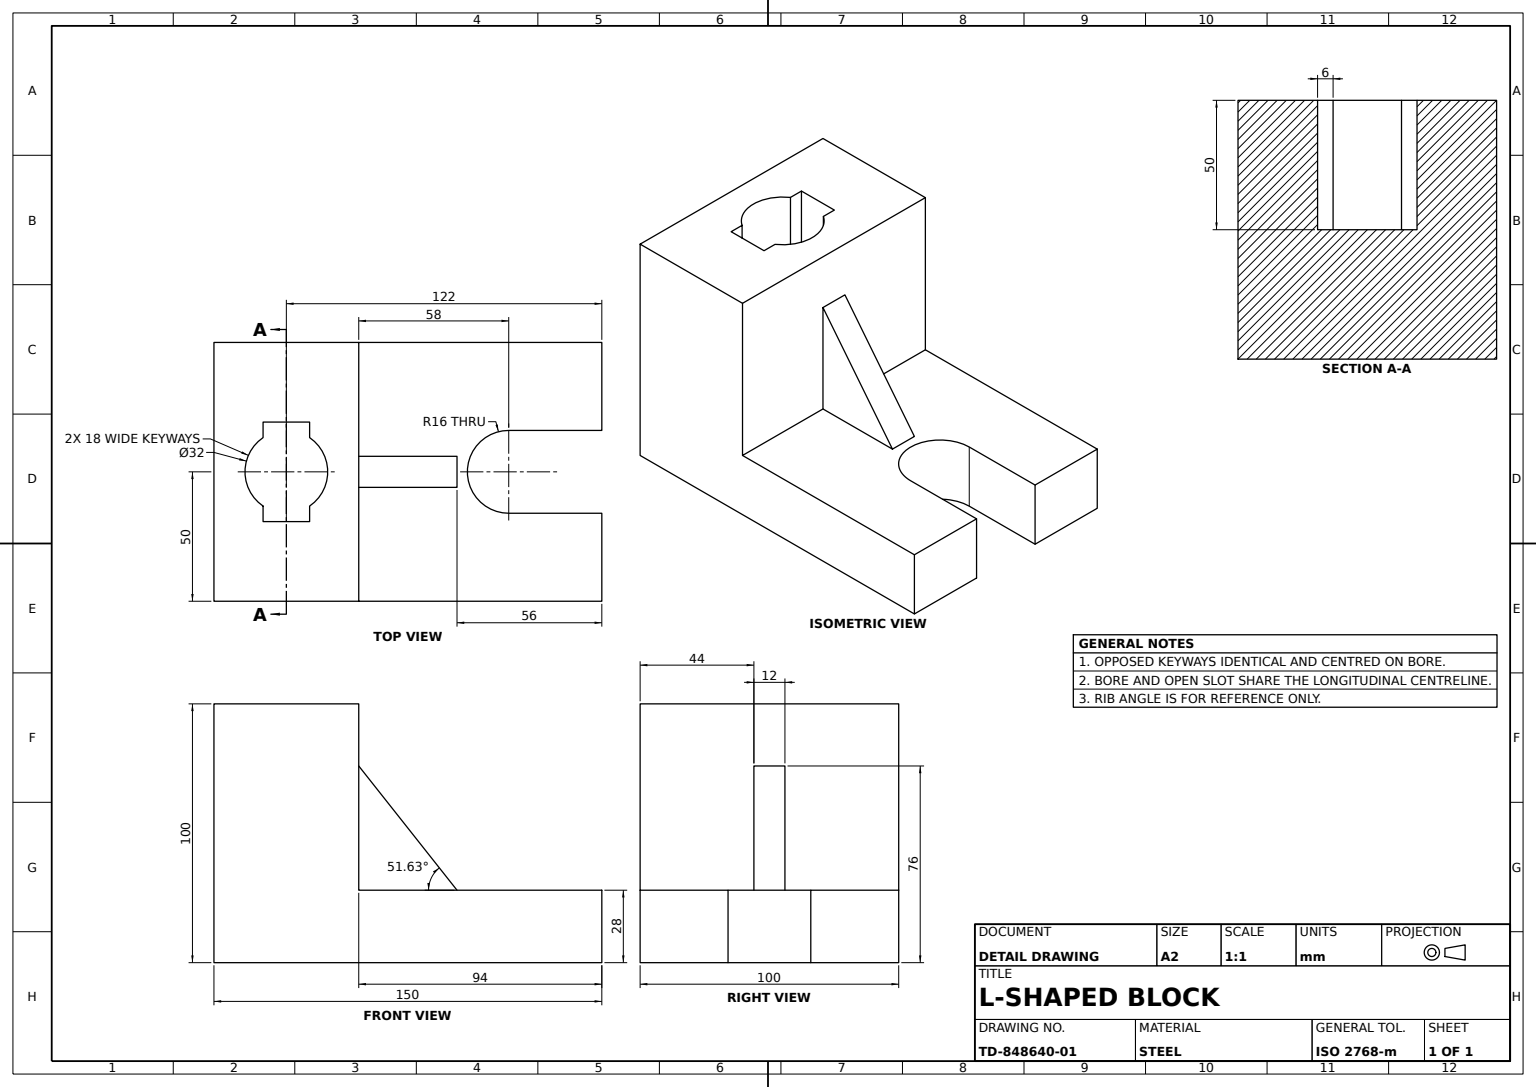
SolidWorks part; units mm, degrees
material "Plain Carbon Steel"
ref_plane "Front Plane" through (0, 0, 0) normal (0, 0, 1) x (1, 0, 0)
ref_plane "Top Plane" through (0, 0, 0) normal (0, 1, 0) x (1, 0, 0)
ref_plane "Right Plane" through (0, 0, 0) normal (1, 0, 0) x (0, 0, -1)
sketch "L-Block Profile Sketch" plane through (0, 0, 0) normal (0, 0, 1) x (1, 0, 0)
  line L0 (0, 0) -> (150, 0)
  line L1 (150, 0) -> (150, 100)
  line L2 (150, 100) -> (94, 100)
  line L3 (0, 0) -> (0, 28)
  line L4 (0, 28) -> (94, 28)
  line L5 (94, 28) -> (94, 100)
  dimension "D1" = 94
  dimension "D2" = 150
  dimension "D3" = 28
  dimension "D4" = 100
extrude "L-Block Base" add sketch "L-Block Profile Sketch" along normal blind 100
sketch "Keyed Bore Sketch" plane through (0, 100, 0) normal (0, 1, 0) x (1, 0, 0)
  line L0 (113, -69.2288) -> (131, -69.2288)
  line L5 (113, -30.7712) -> (113, -36.7712)
  line L6 (131, -30.7712) -> (131, -36.7712)
  line L7 (113, -63.2288) -> (113, -69.2288)
  line L8 (131, -63.2288) -> (131, -69.2288)
  line L9 (113, -30.7712) -> (131, -30.7712)
  arc A0 (113, -36.7712) -> (113, -63.2288) centre (122, -50) ccw
  arc A1 (131, -63.2288) -> (131, -36.7712) centre (122, -50) ccw
  dimension "D1" = 6
  dimension "D5" = 32
  dimension "D2" = 6
  dimension "D3" = 6
  dimension "D4" = 6
  dimension "D6" = 18
  dimension "D7" = 122
  dimension "D8" = 50
extrude "Keyed Bore Cut" cut sketch "Keyed Bore Sketch" against normal blind 50
sketch "Step Boss Sketch" plane through (0, 0, 100) normal (0, 0, 1) x (1, 0, 0)
  line L0 (94, 28) -> (94, 76)
  line L1 (94, 100) -> (94, 28) construction
  line L2 (94, 28) -> (56, 28)
  line L3 (94, 28) -> (0, 28) construction
  line L4 (56, 28) -> (94, 76)
  line L5 (0, 28) -> (0, 0) construction
  line L6 (0, 0) -> (150, 0) construction
  dimension "D1" = 56
  dimension "D2" = 76
extrude "Step Boss" add sketch "Step Boss Sketch" against normal blind 60
sketch "Step Cut Sketch" plane through (0, 0, 100) normal (0, 0, 1) x (1, 0, 0)
  line L0 (94, 76) -> (94, 28)
  line L1 (94, 28) -> (56, 28)
  line L2 (56, 28) -> (0, 28) construction
  line L3 (56, 28) -> (94, 76)
  line L4 (0, 28) -> (0, 0) construction
  dimension "D1" = 56
extrude "Step Cut" cut sketch "Step Cut Sketch" against normal blind 44
sketch "Step Relief Sketch" plane through (0, 0, 40) normal (0, 0, -1) x (-1, 0, 0)
  line L0 (-94, 76) -> (-94, 28)
  line L1 (-56, 28) -> (-94, 28) construction
  line L2 (-94, 28) -> (-94, 76) construction
  line L3 (-94, 28) -> (-56, 28)
  line L4 (-94, 28) -> (0, 28) construction
  line L5 (-56, 28) -> (-94, 76)
extrude "Step Relief Cut" cut sketch "Step Relief Sketch" against normal blind 4
sketch "Low Step Slot Sketch" plane through (0, 28, 0) normal (0, 1, 0) x (1, 0, 0)
  line L0 (0, -34) -> (0, -66)
  line L1 (0, -100) -> (0, 0) construction
  line L2 (36, -34) -> (0, -34)
  line L3 (36, -66) -> (0, -66)
  line L4 (94, -44) -> (94, 0) construction
  line L5 (94, 0) -> (0, 0) construction
  arc A0 (36, -66) -> (36, -34) centre (36, -50) ccw
  dimension "D1" = 16
  dimension "D2" = 58
  dimension "D3" = 50
extrude "Low Step Slot Cut" cut sketch "Low Step Slot Sketch" against normal blind 28
